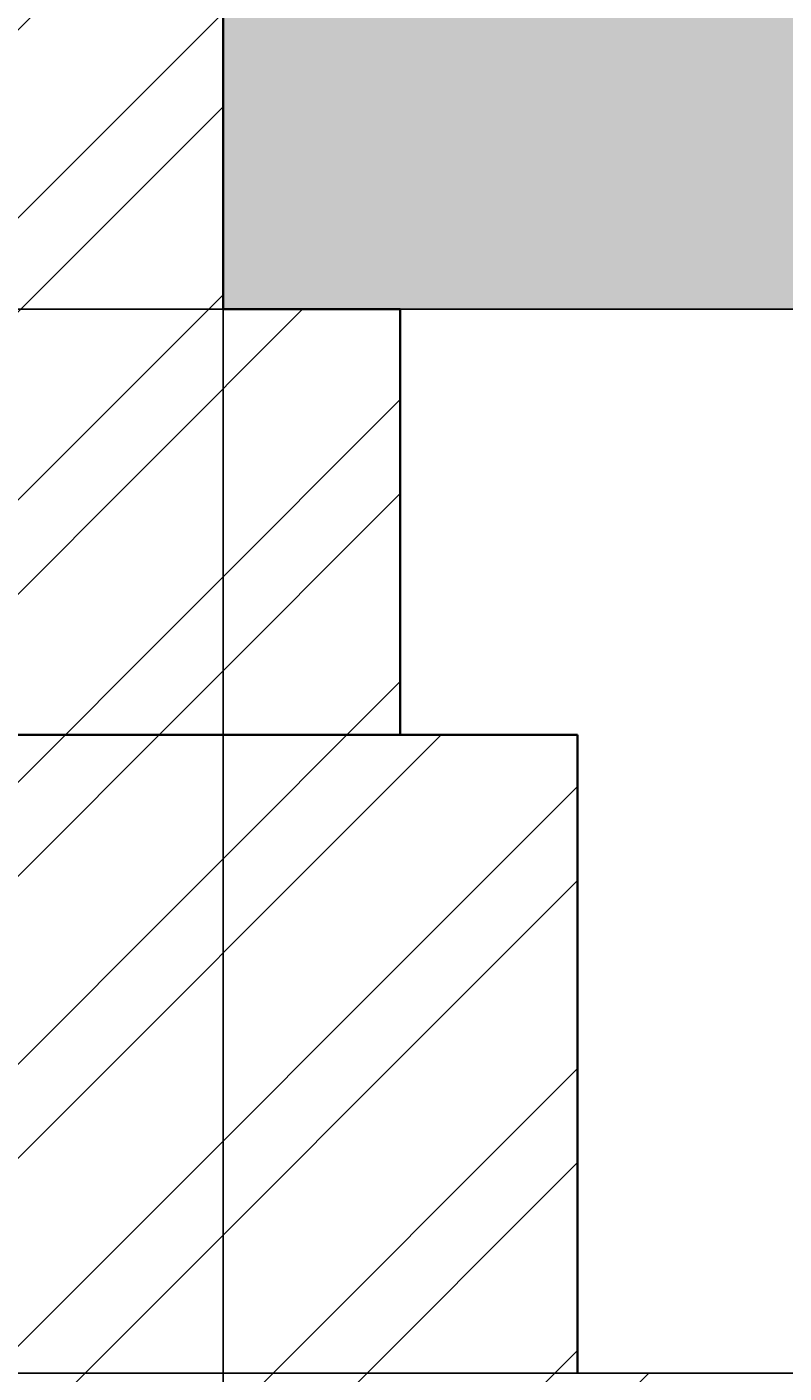
# Model space of a CAD drawing. Units: inches. Extents: x -301 to 715, y -607 to 364.
# Tile 9 of 141: x -41 to -19, y -511 to -474. Entities that reach past the tile are written whole.
import ezdxf

# ---------------------------------------------------------------- set-up
doc = ezdxf.new("R2010")
doc.units = ezdxf.units.IN
doc.header["$MEASUREMENT"] = 0
for name, color, linetype, lineweight in [('A-ANNO-DIMS', 2, 'Continuous', 18), ('A-GRND', 7, 'Continuous', 25), ('A-SECT', 1, 'Continuous', 35), ('A-SECT-PATT', 8, 'Continuous', 13), ('S-FNDN', 2, 'Continuous', 35)]:
    doc.layers.add(name, color=color, linetype=linetype, lineweight=lineweight)
doc.styles.get("Standard").update_dxf_attribs({"font": 'arial.ttf'})
doc.dimstyles.get("Standard").update_dxf_attribs({"dimtxt": 0.18, "dimasz": 0.18, "dimexe": 0.18, "dimexo": 0.0625, "dimgap": 0.09, "dimtad": 0, "dimtih": 1, "dimtoh": 1, "dimdec": 1, "dimzin": 0, "dimdsep": 46, "dimlunit": 4, "dimtxsty": 'Standard', "dimcen": 0.09, "dimclrd": 3, "dimclre": 4, "dimclrt": 6, "dimadec": 0, "dimazin": 0, "dimtfac": 1, "dimtdec": 1, "dimtofl": 0, "dimtmove": 0, "dimatfit": 3, "dimfxl": 1, "dimtfill": 2, "dimtfillclr": 51, "dimtolj": 1, "dimtzin": 0, "dimarcsym": 0})

# ---------------------------------------------------------------- blocks, each defined once
blk = doc.blocks.new('*D179')
at = {"layer": 'A-ANNO-DIMS', "color": 4, "lineweight": -2, "transparency": 16777216}
for p, q in [((-87.981, -433.54), (-87.981, -573.809)), ((-35.282, -463.54), (-35.282, -573.809))]:
    blk.add_line(p, q, dxfattribs=at)
at = {"layer": 'A-ANNO-DIMS', "color": 3, "lineweight": -2, "transparency": 16777216}
for p, q in [((-87.801, -573.629), (-62.174, -573.629)), ((-35.462, -573.629), (-61.089, -573.629))]:
    blk.add_line(p, q, dxfattribs=at)
at = {"layer": 'A-ANNO-DIMS', "color": 3, "transparency": 16777216}
for points in [[(-87.801, -573.599), (-87.801, -573.659), (-87.981, -573.629)], [(-35.462, -573.599), (-35.462, -573.659), (-35.282, -573.629)]]:
    blk.add_solid(points, dxfattribs=at)
at = {"layer": 'Defpoints', "color": 0, "transparency": 16777216}
for p in [(-87.981, -433.477), (-35.282, -463.477), (-35.282, -573.629)]:
    blk.add_point(p, dxfattribs=at)
at = {"layer": 'A-ANNO-DIMS', "color": 6, "transparency": 16777216, "insert": (-61.631, -573.629), "char_height": 0.18, "attachment_point": 5, "bg_fill": 1, "box_fill_scale": 1.25, "bg_fill_color": 51, "bg_fill_transparency": 0}
blk.add_mtext('\\A1;4\'-4 1/2"', dxfattribs=at)
blk = doc.blocks.new('*D180')
at = {"layer": 'A-ANNO-DIMS', "color": 4, "lineweight": -2, "transparency": 16777216}
for p, q in [((-35.282, -463.54), (-35.282, -573.809)), ((12.718, -463.54), (12.718, -573.809))]:
    blk.add_line(p, q, dxfattribs=at)
at = {"layer": 'A-ANNO-DIMS', "color": 3, "lineweight": -2, "transparency": 16777216}
for p, q in [((-35.102, -573.629), (-11.615, -573.629)), ((12.538, -573.629), (-10.949, -573.629))]:
    blk.add_line(p, q, dxfattribs=at)
at = {"layer": 'A-ANNO-DIMS', "color": 3, "transparency": 16777216}
for points in [[(-35.102, -573.599), (-35.102, -573.659), (-35.282, -573.629)], [(12.538, -573.599), (12.538, -573.659), (12.718, -573.629)]]:
    blk.add_solid(points, dxfattribs=at)
at = {"layer": 'Defpoints', "color": 0, "transparency": 16777216}
for p in [(-35.282, -463.477), (12.718, -463.477), (12.718, -573.629)]:
    blk.add_point(p, dxfattribs=at)
at = {"layer": 'A-ANNO-DIMS', "color": 6, "transparency": 16777216, "insert": (-11.282, -573.629), "char_height": 0.18, "attachment_point": 5, "bg_fill": 1, "box_fill_scale": 1.25, "bg_fill_color": 51, "bg_fill_transparency": 0}
blk.add_mtext('\\A1;4\'-0"', dxfattribs=at)
blk = doc.blocks.new('*D190')
at = {"layer": 'A-ANNO-DIMS', "color": 4, "lineweight": -2, "transparency": 16777216}
for p, q in [((129.193, -481.477), (-266.112, -481.477)), ((124.193, -511.477), (-266.112, -511.477))]:
    blk.add_line(p, q, dxfattribs=at)
at = {"layer": 'A-ANNO-DIMS', "color": 3, "lineweight": -2, "transparency": 16777216}
for p, q in [((-265.932, -481.657), (-265.932, -496.296)), ((-265.932, -511.297), (-265.932, -496.659))]:
    blk.add_line(p, q, dxfattribs=at)
at = {"layer": 'A-ANNO-DIMS', "color": 3, "transparency": 16777216}
for points in [[(-265.962, -481.657), (-265.902, -481.657), (-265.932, -481.477)], [(-265.962, -511.297), (-265.902, -511.297), (-265.932, -511.477)]]:
    blk.add_solid(points, dxfattribs=at)
at = {"layer": 'Defpoints', "color": 0, "transparency": 16777216}
for p in [(129.255, -481.477), (-265.932, -511.477), (124.255, -511.477)]:
    blk.add_point(p, dxfattribs=at)
at = {"layer": 'A-ANNO-DIMS', "color": 6, "transparency": 16777216, "insert": (-265.932, -496.477), "char_height": 0.18, "attachment_point": 5, "bg_fill": 1, "box_fill_scale": 1.25, "bg_fill_color": 51, "bg_fill_transparency": 0}
blk.add_mtext('\\A1;2\'-6"', dxfattribs=at)
blk = doc.blocks.new('*D191')
at = {"layer": 'A-ANNO-DIMS', "color": 4, "lineweight": -2, "transparency": 16777216}
for p, q in [((129.193, -481.477), (-266.112, -481.477)), ((114.193, -540.477), (-266.112, -540.477))]:
    blk.add_line(p, q, dxfattribs=at)
at = {"layer": 'A-ANNO-DIMS', "color": 3, "lineweight": -2, "transparency": 16777216}
for p, q in [((-265.932, -481.657), (-265.932, -510.797)), ((-265.932, -540.297), (-265.932, -511.158))]:
    blk.add_line(p, q, dxfattribs=at)
at = {"layer": 'A-ANNO-DIMS', "color": 3, "transparency": 16777216}
for points in [[(-265.962, -481.657), (-265.902, -481.657), (-265.932, -481.477)], [(-265.962, -540.297), (-265.902, -540.297), (-265.932, -540.477)]]:
    blk.add_solid(points, dxfattribs=at)
at = {"layer": 'Defpoints', "color": 0, "transparency": 16777216}
for p in [(129.255, -481.477), (-265.932, -540.477), (114.255, -540.477)]:
    blk.add_point(p, dxfattribs=at)
at = {"layer": 'A-ANNO-DIMS', "color": 6, "transparency": 16777216, "insert": (-265.932, -510.977), "char_height": 0.18, "attachment_point": 5, "bg_fill": 1, "box_fill_scale": 1.25, "bg_fill_color": 51, "bg_fill_transparency": 0}
blk.add_mtext('\\A1;4\'-11"', dxfattribs=at)

msp = doc.modelspace()

# ---------------------------------------------------------------- hatches: boundary and pattern name
at = {"layer": 'A-SECT-PATT'}
h = msp.add_hatch(dxfattribs=at)
h.set_pattern_fill('ANSI32', color=256, scale=15)
h.set_pattern_definition([(45, (10.321, 33.8764), (-3.977476, 3.977476), []), (45, (12.973, 33.8764), (-3.977476, 3.977476), [])])
h.paths.add_polyline_path([(-185.282, -324.477), (-199.282, -324.477), (-199.282, -329.477), (-194.282, -329.477), (-194.282, -353.477), (-185.282, -353.477)])
h.paths.add_polyline_path([(-185.282, -361.477), (-193.904, -361.477), (-193.982, -377.537), (-185.282, -377.537)])
h.paths.add_polyline_path([(143.218, -329.477), (148.218, -329.477), (148.218, -324.477), (134.255, -324.477), (134.255, -353.477), (143.218, -353.477)])
h.paths.add_polyline_path([(143.218, -361.477), (134.255, -361.477), (134.255, -377.477), (143.218, -377.477)])
h.paths.add_polyline_path([(-185.282, -439.477), (-194.282, -439.477), (-194.282, -463.477), (-185.282, -463.477)])
h.paths.add_polyline_path([(-185.282, -471.477), (-194.282, -471.477), (-194.282, -481.477), (-185.282, -481.477)])
h.paths.add_polyline_path([(-185.282, -463.477), (-194.282, -463.477), (-194.282, -466.477), (-185.282, -466.477)])
h.paths.add_polyline_path([(-185.282, -466.477), (-194.282, -466.477), (-194.282, -471.477), (-185.282, -471.477)])
h.paths.add_polyline_path([(-180.282, -481.477), (-185.282, -481.477), (-194.282, -481.477), (-199.282, -481.477), (-199.282, -493.477), (-180.282, -493.477)])
h.paths.add_polyline_path([(-175.282, -493.477), (-180.282, -493.477), (-199.282, -493.477), (-204.282, -493.477), (-204.282, -511.477), (-175.282, -511.477)])
h.paths.add_polyline_path([(-170.282, -511.477), (-175.282, -511.477), (-204.282, -511.477), (-209.282, -511.477), (-209.282, -535.477), (-170.282, -535.477)])
h.paths.add_polyline_path([(-35.282, -463.477), (-41.282, -463.477), (-41.282, -466.477), (-35.282, -466.477)])
h.paths.add_polyline_path([(-35.282, -466.477), (-41.282, -466.477), (-41.282, -471.477), (-35.282, -471.477)])
h.paths.add_polyline_path([(-35.282, -471.477), (-41.282, -471.477), (-41.282, -481.477), (-35.282, -481.477)])
h.paths.add_polyline_path([(-30.282, -481.477), (-46.282, -481.477), (-46.282, -493.477), (-30.282, -493.477)])
h.paths.add_polyline_path([(-25.282, -493.477), (-30.282, -493.477), (-46.282, -493.477), (-51.282, -493.477), (-51.282, -511.477), (-25.282, -511.477)])
h.paths.add_polyline_path([(-20.282, -511.477), (-25.282, -511.477), (-51.282, -511.477), (-56.282, -511.477), (-56.282, -535.477), (-20.282, -535.477)])
h.paths.add_polyline_path([(143.218, -463.477), (134.255, -463.477), (134.255, -466.477), (143.218, -466.477)])
h.paths.add_polyline_path([(143.218, -466.477), (134.255, -466.477), (134.255, -471.477), (143.218, -471.477)])
h.paths.add_polyline_path([(143.218, -471.477), (134.255, -471.477), (134.255, -481.477), (143.218, -481.477)])
h.paths.add_polyline_path([(148.255, -481.477), (143.255, -481.477), (134.255, -481.477), (129.255, -481.477), (129.255, -493.477), (148.255, -493.477)])
h.paths.add_polyline_path([(153.255, -493.477), (148.255, -493.477), (129.255, -493.477), (124.255, -493.477), (124.255, -511.477), (153.255, -511.477)])
h.paths.add_polyline_path([(158.255, -511.477), (153.255, -511.477), (124.255, -511.477), (119.255, -511.477), (119.255, -535.477), (158.255, -535.477)])
h = msp.add_hatch(dxfattribs=at)
h.set_pattern_fill('AR-CONC', color=256, scale=0.5)
h.set_pattern_definition([(50, (10.3213, 33.8764), (3.586301, -0.31376), [0.375, -4.125]), (355, (10.3213, 33.8764), (-0.693757, 3.76096), [0.3, -3.3]), (100.45144, (10.62, 33.8502), (2.892544, 3.4472), [0.3187, -3.50571]), (46.1842, (10.3213, 34.8764), (5.336207, -0.827596), [0.5625, -6.1875]), (96.6356, (10.766, 34.8074), (4.67331, 4.870593), [0.47805, -5.25857]), (351.1842, (10.321, 34.8764), (4.67331, 4.870593), [0.45, -4.95]), (21, (10.8213, 34.6264), (2.984535, -2.013094), [0.375, -4.125]), (326, (10.8213, 34.6264), (1.216577, 3.62575), [0.3, -3.3]), (71.45144, (11.07, 34.4586), (4.201112, 1.612656), [0.3187, -3.50571]), (37.5, (10.3213, 33.8764), (0.0607993, 1.6644693), [0, -3.26, 0, -3.35, 0, -3.3125]), (7.5, (10.3213, 33.8764), (1.3153477, 1.9720586), [0, -1.91, 0, -3.185, 0, -1.2625]), (327.5, (9.2063, 33.8764), (2.6691122, -0.1127744), [0, -1.25, 0, -3.9, 0, -5.175]), (317.5, (8.7063, 33.8764), (2.915931, 0.500525), [0, -1.625, 0, -2.59, 0, -3.675])])
h.paths.add_polyline_path([(-56.282, -535.477), (-61.282, -535.477), (-61.282, -540.477), (-15.282, -540.477), (-15.282, -535.477), (-20.282, -535.477)])
h.paths.add_polyline_path([(119.255, -535.477), (114.255, -535.477), (114.255, -540.477), (163.255, -540.477), (163.255, -535.477), (158.255, -535.477)])
h.paths.add_polyline_path([(-206.282, -471.477), (-209.282, -471.477), (-209.282, -481.477), (-206.282, -481.477), (-194.282, -481.477), (-194.282, -471.477)])
h.paths.add_polyline_path([(-41.282, -481.477), (-41.282, -471.477), (-185.282, -471.477), (-185.282, -481.477), (-180.282, -481.477)])
h.paths.add_polyline_path([(134.255, -481.477), (134.255, -471.477), (-35.282, -471.477), (-35.282, -481.477), (-30.282, -481.477)])
h.paths.add_polyline_path([(155.218, -481.477), (158.218, -481.477), (158.218, -471.477), (153.218, -471.477), (143.218, -471.477), (143.218, -481.477), (148.255, -481.477)])
h.paths.add_polyline_path([(-193.88, -356.477), (-193.904, -361.477), (143.218, -361.477), (143.218, -356.477)])

# ---------------------------------------------------------------- linework, layer by layer
at = {"layer": 'A-GRND'}
msp.add_line((-206.282, -481.477), (155.218, -481.477), dxfattribs=at)
at = {"layer": 'A-SECT'}
msp.add_line((-35.282, -463.477), (-35.282, -481.477), dxfattribs=at)
at = {"layer": 'S-FNDN'}
for p, q in [((-35.282, -481.477), (-30.282, -481.477)), ((-30.282, -481.477), (-30.282, -493.477)), ((-46.282, -493.477), (-30.282, -493.477)), ((-30.282, -493.477), (-25.282, -493.477)), ((-25.282, -493.477), (-25.282, -511.477))]:
    msp.add_line(p, q, dxfattribs=at)

# ---------------------------------------------------------------- dimensions: what is measured, and where the dimension line sits
at = {"layer": 'A-ANNO-DIMS'}
for base, p1, p2, picture, middle in [((-35.282, -573.629), (-87.981, -433.477), (-35.282, -463.477), '*D179', (-61.631, -573.629)), ((12.718, -573.629), (-35.282, -463.477), (12.718, -463.477), '*D180', (-11.282, -573.629))]:
    dim = msp.add_linear_dim(base=base, p1=p1, p2=p2, dimstyle='Standard', override={"dimdec": 1, "dimlfac": 1, "dimrnd": 0, "dimzin": 1, "dimdsep": 46, "dimlunit": 4, "dimfrac": 2}, dxfattribs=at)
    dim.commit()
    dim.dimension.update_dxf_attribs({"geometry": picture, "text_midpoint": middle})
for base, p2, picture, middle in [((-265.932, -540.477), (114.255, -540.477), '*D191', (-265.932, -510.977)), ((-265.932, -511.477), (124.255, -511.477), '*D190', (-265.932, -496.477))]:
    dim = msp.add_linear_dim(base=base, p1=(129.255, -481.477), p2=p2, angle=90, dimstyle='Standard', override={"dimdec": 1, "dimlfac": 1, "dimrnd": 0, "dimzin": 1, "dimdsep": 46, "dimlunit": 4, "dimfrac": 2}, dxfattribs=at)
    dim.commit()
    dim.dimension.update_dxf_attribs({"geometry": picture, "text_midpoint": middle})

doc.saveas('drawing.dxf')
